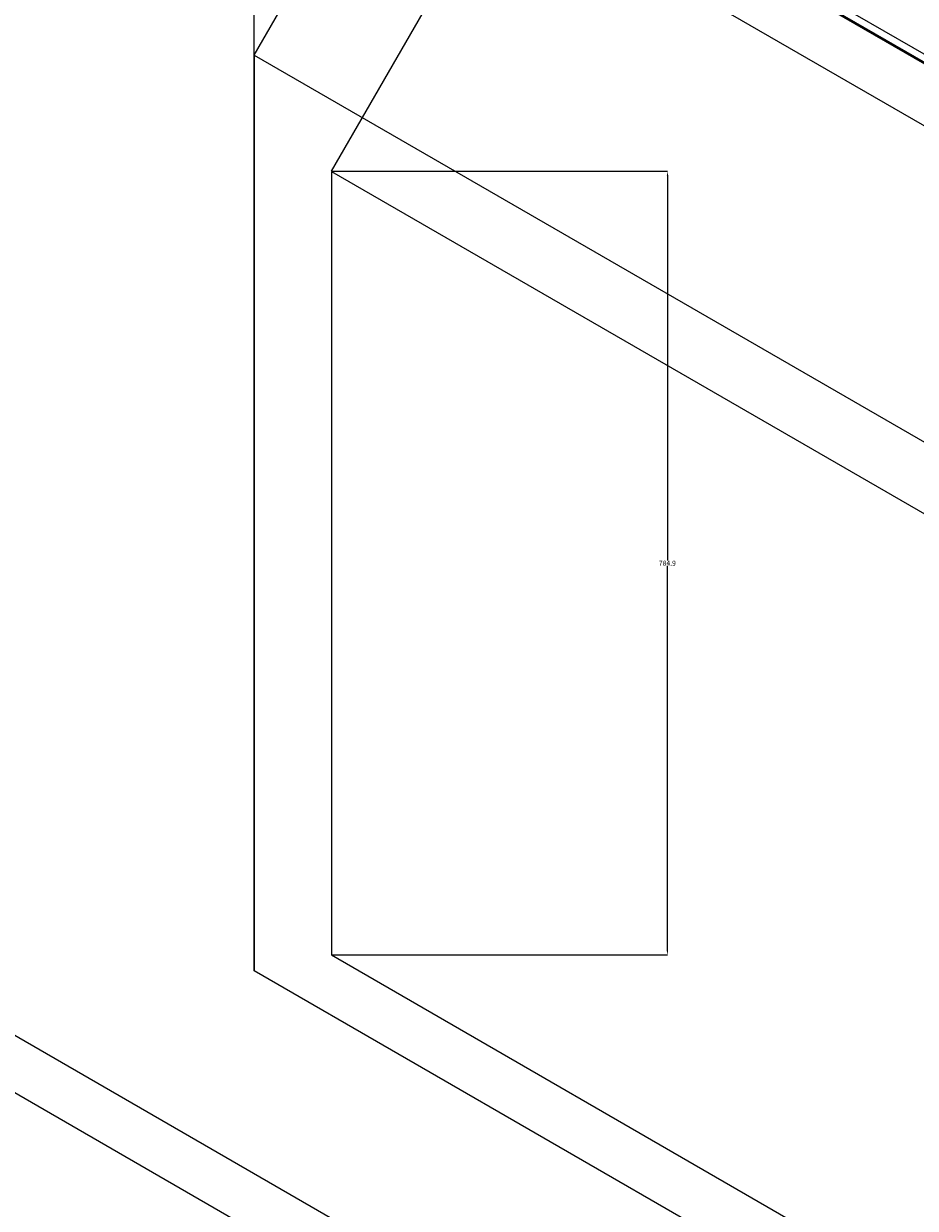
# Model space of a CAD drawing. Units: metres. Extents: x -2391 to 4922, y -635 to 4845.
# Tile 32 of 37: x 1265 to 2158, y 2425 to 3611. Entities that reach past the tile are written whole.
import ezdxf

# ---------------------------------------------------------------- set-up
doc = ezdxf.new("R2010")
doc.units = ezdxf.units.M
doc.header["$MEASUREMENT"] = 0
for name, color, linetype, lineweight in [('A-ANNO-DIMS', 2, 'Continuous', 18), ('A-FLOR-FIXT', 3, 'Continuous', 25), ('A-GLAZ', 4, 'Continuous', 25), ('A-WALL', 7, 'Continuous', 50)]:
    doc.layers.add(name, color=color, linetype=linetype, lineweight=lineweight)
doc.styles.get("Standard").update_dxf_attribs({"font": 'arial.ttf'})
doc.dimstyles.get("Standard").update_dxf_attribs({"dimtxt": 5, "dimasz": 4, "dimexe": 0.18, "dimexo": 0.0625, "dimgap": 0.09, "dimtad": 0, "dimtih": 1, "dimtoh": 1, "dimdec": 0, "dimzin": 0, "dimdsep": 46, "dimtxsty": 'Standard', "dimcen": 0.09, "dimadec": 0, "dimazin": 0, "dimtfac": 1, "dimtdec": 0, "dimtofl": 0, "dimtmove": 0, "dimatfit": 3, "dimfxl": 1, "dimtolj": 1, "dimtzin": 0, "dimarcsym": 0})

# ---------------------------------------------------------------- blocks, each defined once
blk = doc.blocks.new('*D8')
at = {"layer": 'A-ANNO-DIMS', "color": 0, "lineweight": -2, "transparency": 16777216}
for p, q in [((-2047.3, 3005.2), (-2047.3, -631.4)), ((4577.8, 2350.2), (4577.8, -631.4)), ((-2043.3, -631.2), (1257.6, -631.2)), ((4573.8, -631.2), (1272.8, -631.2))]:
    blk.add_line(p, q, dxfattribs=at)
at = {"layer": 'A-ANNO-DIMS', "color": 0, "transparency": 16777216}
for points in [[(-2043.3, -630.6), (-2043.3, -631.9), (-2047.3, -631.2)], [(4573.8, -630.6), (4573.8, -631.9), (4577.8, -631.2)]]:
    blk.add_solid(points, dxfattribs=at)
at = {"layer": 'Defpoints', "color": 0, "transparency": 16777216}
for p in [(-2047.3, 3005.3), (4577.8, 2350.3), (4577.8, -631.2)]:
    blk.add_point(p, dxfattribs=at)
at = {"layer": 'A-ANNO-DIMS', "color": 0, "transparency": 16777216, "insert": (1265.2, -631.2), "char_height": 5, "attachment_point": 5}
blk.add_mtext('\\A1;6625', dxfattribs=at)
blk = doc.blocks.new('*D12')
at = {"layer": 'A-ANNO-DIMS', "color": 0, "lineweight": -2, "transparency": 16777216}
for p, q in [((1496.1, 3579.7), (1664.4, 3871.2)), ((1667.7, 3869), (2357.4, 3470.9)), ((3056.2, 3067.4), (2366.6, 3465.6)), ((2891.5, 2774), (3059.8, 3065.6))]:
    blk.add_line(p, q, dxfattribs=at)
at = {"layer": 'A-ANNO-DIMS', "color": 0, "transparency": 16777216}
for points in [[(1668.1, 3869.6), (1667.4, 3868.5), (1664.3, 3871)], [(3056.6, 3068), (3055.9, 3066.8), (3059.7, 3065.4)]]:
    blk.add_solid(points, dxfattribs=at)
at = {"layer": 'Defpoints', "color": 0, "transparency": 16777216}
for p in [(1496, 3579.6), (3059.7, 3065.4), (2891.4, 2774)]:
    blk.add_point(p, dxfattribs=at)
at = {"layer": 'A-ANNO-DIMS', "color": 0, "transparency": 16777216, "insert": (2362, 3468.2), "char_height": 5, "attachment_point": 5}
blk.add_mtext('\\A1;1611.3', dxfattribs=at)
blk = doc.blocks.new('*D14')
at = {"layer": 'A-ANNO-DIMS', "color": 0, "lineweight": -2, "transparency": 16777216}
for p, q in [((1573.6, 3463.3), (1741.9, 3754.8)), ((1745.2, 3752.7), (2360.9, 3397.3)), ((2985.7, 3036.5), (2370, 3392)), ((2820.9, 2743.2), (2989.2, 3034.7))]:
    blk.add_line(p, q, dxfattribs=at)
at = {"layer": 'A-ANNO-DIMS', "color": 0, "transparency": 16777216}
for points in [[(1745.6, 3753.3), (1744.9, 3752.1), (1741.8, 3754.7)], [(2986, 3037.1), (2985.3, 3036), (2989.1, 3034.5)]]:
    blk.add_solid(points, dxfattribs=at)
at = {"layer": 'Defpoints', "color": 0, "transparency": 16777216}
for p in [(1573.5, 3463.3), (2989.1, 3034.5), (2820.9, 2743.1)]:
    blk.add_point(p, dxfattribs=at)
at = {"layer": 'A-ANNO-DIMS', "color": 0, "transparency": 16777216, "insert": (2365.5, 3394.6), "char_height": 5, "attachment_point": 5}
blk.add_mtext('\\A1;1440.3', dxfattribs=at)
blk = doc.blocks.new('*D15')
at = {"layer": 'A-ANNO-DIMS', "color": 0, "lineweight": -2, "transparency": 16777216}
for p, q in [((1573.6, 3463.3), (1910.2, 3463.3)), ((1910, 3459.3), (1910, 3073.5)), ((1910, 2682.4), (1910, 3068.2)), ((1573.6, 2678.4), (1910.2, 2678.4))]:
    blk.add_line(p, q, dxfattribs=at)
at = {"layer": 'A-ANNO-DIMS', "color": 0, "transparency": 16777216}
for points in [[(1909.4, 3459.3), (1910.7, 3459.3), (1910, 3463.3)], [(1909.4, 2682.4), (1910.7, 2682.4), (1910, 2678.4)]]:
    blk.add_solid(points, dxfattribs=at)
at = {"layer": 'Defpoints', "color": 0, "transparency": 16777216}
for p in [(1573.5, 3463.3), (1573.5, 2678.4), (1910, 2678.4)]:
    blk.add_point(p, dxfattribs=at)
at = {"layer": 'A-ANNO-DIMS', "color": 0, "transparency": 16777216, "insert": (1910, 3070.8), "char_height": 5, "attachment_point": 5}
blk.add_mtext('\\A1;784.9', dxfattribs=at)
blk = doc.blocks.new('*D17')
at = {"layer": 'A-ANNO-DIMS', "color": 0, "lineweight": -2, "transparency": 16777216}
for p, q in [((550.7, 3005.3), (550.7, 4842)), ((554.7, 4841.8), (1014.9, 4841.8)), ((1492, 4841.8), (1031.9, 4841.8)), ((1496, 2662.5), (1496, 4842))]:
    blk.add_line(p, q, dxfattribs=at)
at = {"layer": 'A-ANNO-DIMS', "color": 0, "transparency": 16777216}
for points in [[(554.7, 4842.4), (554.7, 4841.1), (550.7, 4841.8)], [(1492, 4842.4), (1492, 4841.1), (1496, 4841.8)]]:
    blk.add_solid(points, dxfattribs=at)
at = {"layer": 'Defpoints', "color": 0, "transparency": 16777216}
for p in [(1496, 4841.8), (550.7, 3005.3), (1496, 2662.5)]:
    blk.add_point(p, dxfattribs=at)
at = {"layer": 'A-ANNO-DIMS', "color": 0, "transparency": 16777216, "insert": (1023.4, 4841.8), "char_height": 5, "attachment_point": 5}
blk.add_mtext('\\A1;945.3', dxfattribs=at)

msp = doc.modelspace()

# ---------------------------------------------------------------- linework, layer by layer
at = {"layer": 'A-FLOR-FIXT'}
for p, q in [((550.7419, 3005.2763), (3148.8181, 1505.2763)), ((546.8938, 2950.1416), (3148.8181, 1447.9199))]:
    msp.add_line(p, q, dxfattribs=at)
at = {"layer": 'A-GLAZ'}
for p, q in [((1496.0309, 3579.6156), (2891.4324, 2773.9801)), ((1496.0309, 3579.6156), (1496.0309, 2662.4566)), ((1573.5273, 3463.276), (2820.8768, 2743.1184)), ((1573.5273, 3463.276), (1573.5273, 2678.4207)), ((1573.5273, 2678.4207), (2820.8768, 1958.2631)), ((2891.4324, 1856.8211), (1496.0309, 2662.4566))]:
    msp.add_line(p, q, dxfattribs=at)
at = {"layer": 'A-WALL'}
msp.add_line((550.7419, 4505.2763), (3607.8116, 2740.2763), dxfattribs=at)

# ---------------------------------------------------------------- dimensions: what is measured, and where the dimension line sits
at = {"layer": 'A-ANNO-DIMS'}
for base, p1, p2, override, picture, middle in [((1496.0309, 4841.7763), (550.7419, 3005.2763), (1496.0309, 2662.4566), {"dimdec": 1, "dimlfac": 1, "dimrnd": 0, "dimzin": 0, "dimdsep": 46, "dimlunit": 2}, '*D17', (1023.3864, 4841.7763)), ((4577.76, -631.2237), (-2047.3343, 3005.2763), (4577.76, 2350.2763), {"dimdec": 0, "dimlfac": 1, "dimrnd": 0, "dimzin": 0, "dimdsep": 46, "dimlunit": 2}, '*D8', (1265.2128, -631.2237))]:
    dim = msp.add_linear_dim(base=base, p1=p1, p2=p2, dimstyle='Standard', override=override, dxfattribs=at)
    dim.commit()
    dim.dimension.update_dxf_attribs({"geometry": picture, "text_midpoint": middle})
for base, p1, p2, angle, picture, middle in [((3059.6824, 3065.3977), (1496.0309, 3579.6156), (2891.4324, 2773.9801), 330, '*D12', (2361.9817, 3468.2154)), ((2989.1268, 3034.536), (1573.5273, 3463.276), (2820.8768, 2743.1184), 330, '*D14', (2365.4521, 3394.6148)), ((1910.0273, 2678.4207), (1573.5273, 3463.276), (1573.5273, 2678.4207), 270, '*D15', (1910.0273, 3070.8484))]:
    dim = msp.add_linear_dim(base=base, p1=p1, p2=p2, angle=angle, dimstyle='Standard', override={"dimdec": 1, "dimlfac": 1, "dimrnd": 0, "dimzin": 0, "dimdsep": 46, "dimlunit": 2}, dxfattribs=at)
    dim.commit()
    dim.dimension.update_dxf_attribs({"geometry": picture, "text_midpoint": middle})

doc.saveas('drawing.dxf')
